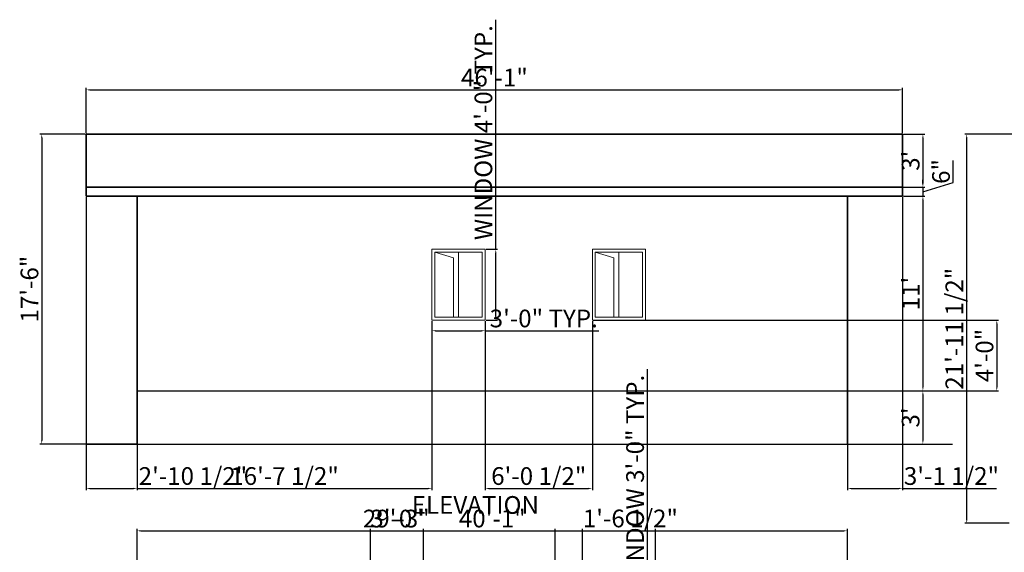
# Model space of a CAD drawing. Units: inches. Extents: x 2319 to 3765, y 2872 to 3950.
# Tile 8 of 9: x 2395 to 3061, y 3589 to 3950. Entities that reach past the tile are written whole.
import ezdxf

# ---------------------------------------------------------------- set-up
doc = ezdxf.new("R2010")
doc.units = ezdxf.units.IN
for name, color, linetype, lineweight in [('A-ANNO-DIMS', 2, 'Continuous', 18), ('A-ANNO-TEXT', 7, 'Continuous', 25), ('A-ELEV', 7, 'Continuous', 25), ('A-GLAZ', 4, 'Continuous', 18), ('A-ROOF', 7, 'Continuous', 35)]:
    doc.layers.add(name, color=color, linetype=linetype, lineweight=lineweight)
doc.styles.get("Standard").update_dxf_attribs({"font": 'arial.ttf'})
doc.dimstyles.new('ISO-25', dxfattribs={"dimtxt": 12, "dimasz": 2.5, "dimexe": 1.25, "dimexo": 0.625, "dimtad": 1, "dimdec": 0, "dimlunit": 3, "dimtxsty": 'Standard', "dimcen": 2.5, "dimadec": 0, "dimazin": 0, "dimtfac": 1, "dimtdec": 0, "dimtmove": 0, "dimatfit": 3, "dimfxl": 1, "dimarcsym": 0})

# ---------------------------------------------------------------- blocks, each defined once
blk = doc.blocks.new('*D27')
at = {"layer": 'A-ANNO-DIMS', "color": 0, "lineweight": -2, "transparency": 16777216}
for p, q in [((2993.13, 3872.56), (3007.48, 3872.56)), ((3006.23, 3870.06), (3006.23, 3839.06)), ((2993.13, 3836.56), (3007.48, 3836.56))]:
    blk.add_line(p, q, dxfattribs=at)
at = {"layer": 'A-ANNO-DIMS', "color": 0, "transparency": 16777216}
for points in [[(3005.82, 3870.06), (3006.65, 3870.06), (3006.23, 3872.56)], [(3005.82, 3839.06), (3006.65, 3839.06), (3006.23, 3836.56)]]:
    blk.add_solid(points, dxfattribs=at)
at = {"layer": 'Defpoints', "color": 0, "transparency": 16777216}
for p in [(2992.5, 3872.56), (2992.5, 3836.56), (3006.23, 3836.56)]:
    blk.add_point(p, dxfattribs=at)
at = {"layer": 'A-ANNO-DIMS', "color": 0, "transparency": 16777216, "insert": (2999.48, 3854.56), "char_height": 12, "attachment_point": 5, "rotation": 90}
blk.add_mtext("3'", dxfattribs=at)
blk = doc.blocks.new('*D28')
at = {"layer": 'A-ANNO-DIMS', "color": 0, "lineweight": -2, "transparency": 16777216}
for p, q in [((3026.8, 3839.73), (3026.8, 3854.84)), ((3006.23, 3839.06), (3006.23, 3841.56)), ((2993.13, 3836.56), (3007.48, 3836.56)), ((3006.23, 3833.56), (3026.8, 3839.73)), ((3006.23, 3836.56), (3006.23, 3830.56)), ((3006.23, 3836.56), (3006.23, 3830.56)), ((2993.13, 3830.56), (3007.48, 3830.56)), ((3006.23, 3828.06), (3006.23, 3825.56))]:
    blk.add_line(p, q, dxfattribs=at)
at = {"layer": 'A-ANNO-DIMS', "color": 0, "transparency": 16777216}
for points in [[(3005.82, 3839.06), (3006.65, 3839.06), (3006.23, 3836.56)], [(3005.82, 3828.06), (3006.65, 3828.06), (3006.23, 3830.56)]]:
    blk.add_solid(points, dxfattribs=at)
at = {"layer": 'Defpoints', "color": 0, "transparency": 16777216}
for p in [(2992.5, 3836.56), (2992.5, 3830.56), (3006.23, 3830.56)]:
    blk.add_point(p, dxfattribs=at)
at = {"layer": 'A-ANNO-DIMS', "color": 0, "transparency": 16777216, "insert": (3020.05, 3847.29), "char_height": 12, "attachment_point": 5, "rotation": 90}
blk.add_mtext('6"', dxfattribs=at)
blk = doc.blocks.new('*D29')
at = {"layer": 'A-ANNO-DIMS', "color": 0, "lineweight": -2, "transparency": 16777216}
for p, q in [((2993.13, 3830.56), (3007.48, 3830.56)), ((3006.23, 3828.06), (3006.23, 3701.06)), ((2955.75, 3698.56), (3007.48, 3698.56))]:
    blk.add_line(p, q, dxfattribs=at)
at = {"layer": 'A-ANNO-DIMS', "color": 0, "transparency": 16777216}
for points in [[(3005.82, 3828.06), (3006.65, 3828.06), (3006.23, 3830.56)], [(3005.82, 3701.06), (3006.65, 3701.06), (3006.23, 3698.56)]]:
    blk.add_solid(points, dxfattribs=at)
at = {"layer": 'Defpoints', "color": 0, "transparency": 16777216}
for p in [(2992.5, 3830.56), (2955.13, 3698.56), (3006.23, 3698.56)]:
    blk.add_point(p, dxfattribs=at)
at = {"layer": 'A-ANNO-DIMS', "color": 0, "transparency": 16777216, "insert": (2999.58, 3764.56), "char_height": 12, "attachment_point": 5, "rotation": 90}
blk.add_mtext("11'", dxfattribs=at)
blk = doc.blocks.new('*D30')
at = {"layer": 'A-ANNO-DIMS', "color": 0, "lineweight": -2, "transparency": 16777216}
for p, q in [((2955.75, 3698.56), (3007.48, 3698.56)), ((3006.23, 3696.06), (3006.23, 3665.06)), ((2955.75, 3662.56), (3007.48, 3662.56))]:
    blk.add_line(p, q, dxfattribs=at)
at = {"layer": 'A-ANNO-DIMS', "color": 0, "transparency": 16777216}
for points in [[(3005.82, 3696.06), (3006.65, 3696.06), (3006.23, 3698.56)], [(3005.82, 3665.06), (3006.65, 3665.06), (3006.23, 3662.56)]]:
    blk.add_solid(points, dxfattribs=at)
at = {"layer": 'Defpoints', "color": 0, "transparency": 16777216}
for p in [(2955.13, 3698.56), (2955.13, 3662.56), (3006.23, 3662.56)]:
    blk.add_point(p, dxfattribs=at)
at = {"layer": 'A-ANNO-DIMS', "color": 0, "transparency": 16777216, "insert": (2999.48, 3680.56), "char_height": 12, "attachment_point": 5, "rotation": 90}
blk.add_mtext("3'", dxfattribs=at)
blk = doc.blocks.new('WIN-36X48-ELEV')
for p, q in [((2, 46), (14.59, 42.21)), ((14.59, 42.21), (14.59, 2.09)), ((18, 2), (18, 46))]:
    blk.add_line(p, q)
for points in [[(0, 0), (36, 0), (36, 48), (0, 48)], [(2, 2), (34, 2), (34, 46), (2, 46)]]:
    blk.add_lwpolyline(points, close=True)
blk = doc.blocks.new('*D61')
at = {"layer": 'A-ANNO-DIMS', "color": 0, "lineweight": -2, "transparency": 16777216}
for p, q in [((2819.73, 3557.62), (2819.73, 3713.22)), ((2824.5, 3557.62), (2818.48, 3557.62)), ((2819.73, 3524.12), (2819.73, 3555.12)), ((2824.5, 3521.62), (2818.48, 3521.62))]:
    blk.add_line(p, q, dxfattribs=at)
at = {"layer": 'A-ANNO-DIMS', "color": 0, "transparency": 16777216}
for points in [[(2819.31, 3555.12), (2820.14, 3555.12), (2819.73, 3557.62)], [(2819.31, 3524.12), (2820.14, 3524.12), (2819.73, 3521.62)]]:
    blk.add_solid(points, dxfattribs=at)
at = {"layer": 'Defpoints', "color": 0, "transparency": 16777216}
for p in [(2819.73, 3557.62), (2825.13, 3557.62), (2825.13, 3521.62)]:
    blk.add_point(p, dxfattribs=at)
at = {"layer": 'A-ANNO-DIMS', "color": 0, "transparency": 16777216, "insert": (2812.89, 3636.67), "char_height": 12, "attachment_point": 5, "rotation": 90}
blk.add_mtext('WINDOW 3\'-0" TYP.', dxfattribs=at)
blk = doc.blocks.new('*D67')
at = {"layer": 'A-ANNO-DIMS', "color": 0, "lineweight": -2, "transparency": 16777216}
for p, q in [((2717.01, 3794.56), (2717.01, 3950.16)), ((2710.44, 3794.56), (2718.26, 3794.56)), ((2717.01, 3749.06), (2717.01, 3792.06)), ((2710.44, 3746.56), (2718.26, 3746.56))]:
    blk.add_line(p, q, dxfattribs=at)
at = {"layer": 'A-ANNO-DIMS', "color": 0, "transparency": 16777216}
for points in [[(2716.6, 3792.06), (2717.43, 3792.06), (2717.01, 3794.56)], [(2716.6, 3749.06), (2717.43, 3749.06), (2717.01, 3746.56)]]:
    blk.add_solid(points, dxfattribs=at)
at = {"layer": 'Defpoints', "color": 0, "transparency": 16777216}
for p in [(2709.81, 3794.56), (2717.01, 3794.56), (2709.81, 3746.56)]:
    blk.add_point(p, dxfattribs=at)
at = {"layer": 'A-ANNO-DIMS', "color": 0, "transparency": 16777216, "insert": (2710.18, 3873.61), "char_height": 12, "attachment_point": 5, "rotation": 90}
blk.add_mtext('WINDOW 4\'-0" TYP.', dxfattribs=at)
blk = doc.blocks.new('*D68')
at = {"layer": 'A-ANNO-DIMS', "color": 0, "lineweight": -2, "transparency": 16777216}
for p, q in [((2673.81, 3745.94), (2673.81, 3738.11)), ((2709.81, 3745.94), (2709.81, 3738.11)), ((2676.31, 3739.36), (2707.31, 3739.36)), ((2709.81, 3739.36), (2786.7, 3739.36))]:
    blk.add_line(p, q, dxfattribs=at)
at = {"layer": 'A-ANNO-DIMS', "color": 0, "transparency": 16777216}
for points in [[(2676.31, 3739.78), (2676.31, 3738.94), (2673.81, 3739.36)], [(2707.31, 3739.78), (2707.31, 3738.94), (2709.81, 3739.36)]]:
    blk.add_solid(points, dxfattribs=at)
at = {"layer": 'Defpoints', "color": 0, "transparency": 16777216}
for p in [(2673.81, 3746.56), (2709.81, 3746.56), (2709.81, 3739.36)]:
    blk.add_point(p, dxfattribs=at)
at = {"layer": 'A-ANNO-DIMS', "color": 0, "transparency": 16777216, "insert": (2749.51, 3746.12), "char_height": 12, "attachment_point": 5}
blk.add_mtext('3\'-0" TYP.', dxfattribs=at)
blk = doc.blocks.new('*D71')
at = {"layer": 'A-ANNO-DIMS', "color": 0, "lineweight": -2, "transparency": 16777216}
for p, q in [((2474.13, 3507.24), (2474.13, 3605.01)), ((2476.63, 3603.76), (2952.63, 3603.76)), ((2955.13, 3569.24), (2955.13, 3605.01))]:
    blk.add_line(p, q, dxfattribs=at)
at = {"layer": 'A-ANNO-DIMS', "color": 0, "transparency": 16777216}
for points in [[(2476.63, 3604.18), (2476.63, 3603.34), (2474.13, 3603.76)], [(2952.63, 3604.18), (2952.63, 3603.34), (2955.13, 3603.76)]]:
    blk.add_solid(points, dxfattribs=at)
at = {"layer": 'Defpoints', "color": 0, "transparency": 16777216}
for p in [(2955.13, 3603.76), (2955.13, 3568.61), (2474.13, 3506.61)]:
    blk.add_point(p, dxfattribs=at)
at = {"layer": 'A-ANNO-DIMS', "color": 0, "transparency": 16777216, "insert": (2714.63, 3610.51), "char_height": 12, "attachment_point": 5}
blk.add_mtext('40\'-1"', dxfattribs=at)
blk = doc.blocks.new('*D73')
at = {"layer": 'A-ANNO-DIMS', "color": 0, "lineweight": -2, "transparency": 16777216}
for p, q in [((2474.13, 3507.24), (2474.13, 3605.01)), ((2476.63, 3603.76), (2822.63, 3603.76)), ((2825.13, 3507.24), (2825.13, 3605.01))]:
    blk.add_line(p, q, dxfattribs=at)
at = {"layer": 'A-ANNO-DIMS', "color": 0, "transparency": 16777216}
for points in [[(2476.63, 3604.18), (2476.63, 3603.34), (2474.13, 3603.76)], [(2822.63, 3604.18), (2822.63, 3603.34), (2825.13, 3603.76)]]:
    blk.add_solid(points, dxfattribs=at)
at = {"layer": 'Defpoints', "color": 0, "transparency": 16777216}
for p in [(2825.13, 3603.76), (2474.13, 3506.61), (2825.13, 3506.61)]:
    blk.add_point(p, dxfattribs=at)
at = {"layer": 'A-ANNO-DIMS', "color": 0, "transparency": 16777216, "insert": (2649.63, 3610.52), "char_height": 12, "attachment_point": 5}
blk.add_mtext('29\'-3"', dxfattribs=at)
blk = doc.blocks.new('*D75')
at = {"layer": 'A-ANNO-DIMS', "color": 0, "lineweight": -2, "transparency": 16777216}
for p, q in [((2632.13, 2970.24), (2632.13, 3605.01)), ((2634.63, 3603.76), (2665.63, 3603.76)), ((2668.13, 2970.24), (2668.13, 3605.01))]:
    blk.add_line(p, q, dxfattribs=at)
at = {"layer": 'A-ANNO-DIMS', "color": 0, "transparency": 16777216}
for points in [[(2634.63, 3604.18), (2634.63, 3603.34), (2632.13, 3603.76)], [(2665.63, 3604.18), (2665.63, 3603.34), (2668.13, 3603.76)]]:
    blk.add_solid(points, dxfattribs=at)
at = {"layer": 'Defpoints', "color": 0, "transparency": 16777216}
for p in [(2668.13, 3603.76), (2632.13, 2969.61), (2668.13, 2969.61)]:
    blk.add_point(p, dxfattribs=at)
at = {"layer": 'A-ANNO-DIMS', "color": 0, "transparency": 16777216, "insert": (2650.13, 3610.52), "char_height": 12, "attachment_point": 5}
blk.add_mtext('3\'-0"', dxfattribs=at)
blk = doc.blocks.new('*D76')
at = {"layer": 'A-ANNO-DIMS', "color": 0, "lineweight": -2, "transparency": 16777216}
for p, q in [((2757.13, 2970.24), (2757.13, 3605.01)), ((2759.63, 3603.76), (2773.17, 3603.76)), ((2775.67, 2970.24), (2775.67, 3605.01)), ((2775.67, 3603.76), (2838.15, 3603.76))]:
    blk.add_line(p, q, dxfattribs=at)
at = {"layer": 'A-ANNO-DIMS', "color": 0, "transparency": 16777216}
for points in [[(2759.63, 3604.18), (2759.63, 3603.34), (2757.13, 3603.76)], [(2773.17, 3604.18), (2773.17, 3603.34), (2775.67, 3603.76)]]:
    blk.add_solid(points, dxfattribs=at)
at = {"layer": 'Defpoints', "color": 0, "transparency": 16777216}
for p in [(2775.67, 3603.76), (2757.13, 2969.61), (2775.67, 2969.61)]:
    blk.add_point(p, dxfattribs=at)
at = {"layer": 'A-ANNO-DIMS', "color": 0, "transparency": 16777216, "insert": (2808.16, 3610.59), "char_height": 12, "attachment_point": 5}
blk.add_mtext('1\'-6 1/2"', dxfattribs=at)
blk = doc.blocks.new('*D89')
at = {"layer": 'A-ANNO-DIMS', "color": 0, "lineweight": -2, "transparency": 16777216}
for p, q in [((2439.63, 3873.19), (2439.63, 3903.86)), ((2442.13, 3902.61), (2990, 3902.61)), ((2992.5, 3873.19), (2992.5, 3903.86))]:
    blk.add_line(p, q, dxfattribs=at)
at = {"layer": 'A-ANNO-DIMS', "color": 0, "transparency": 16777216}
for points in [[(2442.13, 3903.03), (2442.13, 3902.19), (2439.63, 3902.61)], [(2990, 3903.03), (2990, 3902.19), (2992.5, 3902.61)]]:
    blk.add_solid(points, dxfattribs=at)
at = {"layer": 'Defpoints', "color": 0, "transparency": 16777216}
for p in [(2992.5, 3902.61), (2439.63, 3872.56), (2992.5, 3872.56)]:
    blk.add_point(p, dxfattribs=at)
at = {"layer": 'A-ANNO-DIMS', "color": 0, "transparency": 16777216, "insert": (2716.07, 3909.36), "char_height": 12, "attachment_point": 5}
blk.add_mtext('46\'-1"', dxfattribs=at)
blk = doc.blocks.new('*D90')
at = {"layer": 'A-ANNO-DIMS', "color": 0, "lineweight": -2, "transparency": 16777216}
for p, q in [((2439, 3872.56), (2408.33, 3872.56)), ((2409.58, 3870.06), (2409.58, 3665.06)), ((2473.5, 3662.56), (2408.33, 3662.56))]:
    blk.add_line(p, q, dxfattribs=at)
at = {"layer": 'A-ANNO-DIMS', "color": 0, "transparency": 16777216}
for points in [[(2409.16, 3870.06), (2409.99, 3870.06), (2409.58, 3872.56)], [(2409.16, 3665.06), (2409.99, 3665.06), (2409.58, 3662.56)]]:
    blk.add_solid(points, dxfattribs=at)
at = {"layer": 'Defpoints', "color": 0, "transparency": 16777216}
for p in [(2439.63, 3872.56), (2409.58, 3662.56), (2474.13, 3662.56)]:
    blk.add_point(p, dxfattribs=at)
at = {"layer": 'A-ANNO-DIMS', "color": 0, "transparency": 16777216, "insert": (2402.83, 3767.56), "char_height": 12, "attachment_point": 5, "rotation": 90}
blk.add_mtext('17\'-6"', dxfattribs=at)
blk = doc.blocks.new('*D91')
at = {"layer": 'A-ANNO-DIMS', "color": 0, "lineweight": -2, "transparency": 16777216}
for p, q in [((2439.63, 3829.94), (2439.63, 3631.26)), ((2474.13, 3829.94), (2474.13, 3631.26)), ((2442.13, 3632.51), (2471.63, 3632.51)), ((2474.13, 3632.51), (2547.27, 3632.51))]:
    blk.add_line(p, q, dxfattribs=at)
at = {"layer": 'A-ANNO-DIMS', "color": 0, "transparency": 16777216}
for points in [[(2442.13, 3632.93), (2442.13, 3632.09), (2439.63, 3632.51)], [(2471.63, 3632.93), (2471.63, 3632.09), (2474.13, 3632.51)]]:
    blk.add_solid(points, dxfattribs=at)
at = {"layer": 'Defpoints', "color": 0, "transparency": 16777216}
for p in [(2439.63, 3830.56), (2474.13, 3830.56), (2474.13, 3632.51)]:
    blk.add_point(p, dxfattribs=at)
at = {"layer": 'A-ANNO-DIMS', "color": 0, "transparency": 16777216, "insert": (2511.95, 3639.34), "char_height": 12, "attachment_point": 5}
blk.add_mtext('2\'-10 1/2"', dxfattribs=at)
blk = doc.blocks.new('*D92')
at = {"layer": 'A-ANNO-DIMS', "color": 0, "lineweight": -2, "transparency": 16777216}
for p, q in [((2955.13, 3829.94), (2955.13, 3631.26)), ((2992.5, 3829.94), (2992.5, 3631.26)), ((2957.63, 3632.51), (2990, 3632.51)), ((2992.5, 3632.51), (3056.11, 3632.51))]:
    blk.add_line(p, q, dxfattribs=at)
at = {"layer": 'A-ANNO-DIMS', "color": 0, "transparency": 16777216}
for points in [[(2957.63, 3632.93), (2957.63, 3632.09), (2955.13, 3632.51)], [(2990, 3632.93), (2990, 3632.09), (2992.5, 3632.51)]]:
    blk.add_solid(points, dxfattribs=at)
at = {"layer": 'Defpoints', "color": 0, "transparency": 16777216}
for p in [(2955.13, 3830.56), (2992.5, 3830.56), (2992.5, 3632.51)]:
    blk.add_point(p, dxfattribs=at)
at = {"layer": 'A-ANNO-DIMS', "color": 0, "transparency": 16777216, "insert": (3025.56, 3639.34), "char_height": 12, "attachment_point": 5}
blk.add_mtext('3\'-1 1/2"', dxfattribs=at)
blk = doc.blocks.new('*D93')
at = {"layer": 'A-ANNO-DIMS', "color": 0, "lineweight": -2, "transparency": 16777216}
for p, q in [((2673.81, 3745.94), (2673.81, 3631.26)), ((2474.13, 3697.94), (2474.13, 3631.26)), ((2476.63, 3632.51), (2671.31, 3632.51))]:
    blk.add_line(p, q, dxfattribs=at)
at = {"layer": 'A-ANNO-DIMS', "color": 0, "transparency": 16777216}
for points in [[(2476.63, 3632.93), (2476.63, 3632.09), (2474.13, 3632.51)], [(2671.31, 3632.93), (2671.31, 3632.09), (2673.81, 3632.51)]]:
    blk.add_solid(points, dxfattribs=at)
at = {"layer": 'Defpoints', "color": 0, "transparency": 16777216}
for p in [(2673.81, 3746.56), (2474.13, 3698.56), (2673.81, 3632.51)]:
    blk.add_point(p, dxfattribs=at)
at = {"layer": 'A-ANNO-DIMS', "color": 0, "transparency": 16777216, "insert": (2573.97, 3639.34), "char_height": 12, "attachment_point": 5}
blk.add_mtext('16\'-7 1/2"', dxfattribs=at)
blk = doc.blocks.new('*D94')
at = {"layer": 'A-ANNO-DIMS', "color": 0, "lineweight": -2, "transparency": 16777216}
for p, q in [((2709.81, 3745.94), (2709.81, 3631.26)), ((2782.41, 3745.94), (2782.41, 3631.26)), ((2712.31, 3632.51), (2779.91, 3632.51))]:
    blk.add_line(p, q, dxfattribs=at)
at = {"layer": 'A-ANNO-DIMS', "color": 0, "transparency": 16777216}
for points in [[(2712.31, 3632.93), (2712.31, 3632.09), (2709.81, 3632.51)], [(2779.91, 3632.93), (2779.91, 3632.09), (2782.41, 3632.51)]]:
    blk.add_solid(points, dxfattribs=at)
at = {"layer": 'Defpoints', "color": 0, "transparency": 16777216}
for p in [(2709.81, 3746.56), (2782.41, 3746.56), (2782.41, 3632.51)]:
    blk.add_point(p, dxfattribs=at)
at = {"layer": 'A-ANNO-DIMS', "color": 0, "transparency": 16777216, "insert": (2746.11, 3639.34), "char_height": 12, "attachment_point": 5}
blk.add_mtext('6\'-0 1/2"', dxfattribs=at)
blk = doc.blocks.new('*D95')
at = {"layer": 'A-ANNO-DIMS', "color": 0, "lineweight": -2, "transparency": 16777216}
for p, q in [((2783.03, 3746.56), (3057.51, 3746.56)), ((3056.26, 3744.06), (3056.26, 3701.06)), ((2955.75, 3698.56), (3057.51, 3698.56))]:
    blk.add_line(p, q, dxfattribs=at)
at = {"layer": 'A-ANNO-DIMS', "color": 0, "transparency": 16777216}
for points in [[(3055.84, 3744.06), (3056.67, 3744.06), (3056.26, 3746.56)], [(3055.84, 3701.06), (3056.67, 3701.06), (3056.26, 3698.56)]]:
    blk.add_solid(points, dxfattribs=at)
at = {"layer": 'Defpoints', "color": 0, "transparency": 16777216}
for p in [(2782.41, 3746.56), (2955.13, 3698.56), (3056.26, 3698.56)]:
    blk.add_point(p, dxfattribs=at)
at = {"layer": 'A-ANNO-DIMS', "color": 0, "transparency": 16777216, "insert": (3049.5, 3722.56), "char_height": 12, "attachment_point": 5, "rotation": 90}
blk.add_mtext('4\'-0"', dxfattribs=at)
blk = doc.blocks.new('*D97')
at = {"layer": 'A-ANNO-DIMS', "color": 0, "lineweight": -2, "transparency": 16777216}
for p, q in [((3077.94, 3872.56), (3034.65, 3872.56)), ((3035.9, 3611.36), (3035.9, 3870.06)), ((3064.57, 3608.86), (3034.65, 3608.86))]:
    blk.add_line(p, q, dxfattribs=at)
at = {"layer": 'A-ANNO-DIMS', "color": 0, "transparency": 16777216}
for points in [[(3035.48, 3870.06), (3036.31, 3870.06), (3035.9, 3872.56)], [(3035.48, 3611.36), (3036.31, 3611.36), (3035.9, 3608.86)]]:
    blk.add_solid(points, dxfattribs=at)
at = {"layer": 'Defpoints', "color": 0, "transparency": 16777216}
for p in [(3035.9, 3872.56), (3078.57, 3872.56), (3065.2, 3608.86)]:
    blk.add_point(p, dxfattribs=at)
at = {"layer": 'A-ANNO-DIMS', "color": 0, "transparency": 16777216, "insert": (3029.07, 3740.71), "char_height": 12, "attachment_point": 5, "rotation": 90}
blk.add_mtext('21\'-11 1/2"', dxfattribs=at)

msp = doc.modelspace()

# ---------------------------------------------------------------- linework, layer by layer
at = {"layer": 'A-ELEV'}
for p, q in [((2474.13, 3662.56), (2474.13, 3830.56)), ((2955.13, 3662.56), (2955.13, 3830.56)), ((2474.13, 3698.56), (2955.13, 3698.56)), ((2439.63, 3662.56), (3026.21, 3662.56))]:
    msp.add_line(p, q, dxfattribs=at)
at = {"layer": 'A-ROOF'}
for p, q in [((2439.63, 3872.56), (2992.5, 3872.56)), ((2439.63, 3830.56), (2439.63, 3872.56)), ((2992.5, 3830.56), (2992.5, 3872.56)), ((2439.63, 3836.56), (2992.5, 3836.56)), ((2439.63, 3830.56), (2992.5, 3830.56))]:
    msp.add_line(p, q, dxfattribs=at)

# ---------------------------------------------------------------- block references
at = {"layer": 'A-GLAZ'}
for p in [(2673.81, 3746.56), (2782.41, 3746.56)]:
    msp.add_blockref('WIN-36X48-ELEV', p, dxfattribs=at)

# ---------------------------------------------------------------- texts
at = {"layer": 'A-ANNO-TEXT'}
msp.add_text('ELEVATION', height=12, dxfattribs=at).set_placement((2660.13, 3615.29))

# ---------------------------------------------------------------- dimensions: what is measured, and where the dimension line sits
at = {"layer": 'A-ANNO-DIMS'}
for base, p1, p2, picture, middle in [((2717.01, 3794.56), (2709.81, 3746.56), (2709.81, 3794.56), '*D67', (2710.18, 3873.61)), ((2819.73, 3557.62), (2825.13, 3521.62), (2825.13, 3557.62), '*D61', (2812.89, 3636.67))]:
    dim = msp.add_linear_dim(base=base, p1=p1, p2=p2, angle=90, text='WINDOW <> TYP.', dimstyle='ISO-25', override={"dimdec": 1, "dimlfac": 1, "dimrnd": 0, "dimzin": 1, "dimdsep": 46, "dimlunit": 4, "dimfrac": 2}, dxfattribs=at)
    dim.commit()
    dim.dimension.update_dxf_attribs({"geometry": picture, "text_midpoint": middle})
for base, p1, p2, picture, middle in [((2992.5, 3902.61), (2439.63, 3872.56), (2992.5, 3872.56), '*D89', (2716.07, 3909.36)), ((2474.13, 3632.51), (2439.63, 3830.56), (2474.13, 3830.56), '*D91', (2511.95, 3639.34)), ((2992.5, 3632.51), (2955.13, 3830.56), (2992.5, 3830.56), '*D92', (3025.56, 3639.34)), ((2673.81, 3632.51), (2474.13, 3698.56), (2673.81, 3746.56), '*D93', (2573.97, 3639.34)), ((2782.41, 3632.51), (2709.81, 3746.56), (2782.41, 3746.56), '*D94', (2746.11, 3639.34)), ((2775.67, 3603.76), (2757.13, 2969.61), (2775.67, 2969.61), '*D76', (2808.16, 3610.59)), ((2955.13, 3603.76), (2474.13, 3506.61), (2955.13, 3568.61), '*D71', (2714.63, 3610.51)), ((2825.13, 3603.76), (2474.13, 3506.61), (2825.13, 3506.61), '*D73', (2649.63, 3610.52)), ((2668.13, 3603.76), (2632.13, 2969.61), (2668.13, 2969.61), '*D75', (2650.13, 3610.52))]:
    dim = msp.add_linear_dim(base=base, p1=p1, p2=p2, dimstyle='ISO-25', override={"dimdec": 1, "dimlfac": 1, "dimrnd": 0, "dimzin": 1, "dimdsep": 46, "dimlunit": 4, "dimfrac": 2}, dxfattribs=at)
    dim.commit()
    dim.dimension.update_dxf_attribs({"geometry": picture, "text_midpoint": middle})
for base, p1, p2, override, picture, middle in [((2409.58, 3662.56), (2439.63, 3872.56), (2474.13, 3662.56), {"dimdec": 1, "dimlfac": 1, "dimrnd": 0, "dimzin": 1, "dimdsep": 46, "dimlunit": 4, "dimfrac": 2}, '*D90', (2402.83, 3767.56)), ((3006.23, 3836.56), (2992.5, 3872.56), (2992.5, 3836.56), {"dimclrd": 0, "dimclre": 0, "dimclrt": 0}, '*D27', (2999.48, 3854.56)), ((3035.9, 3872.56), (3065.2, 3608.86), (3078.57, 3872.56), {"dimdec": 1, "dimlfac": 1, "dimrnd": 0, "dimzin": 1, "dimdsep": 46, "dimlunit": 4, "dimfrac": 2}, '*D97', (3029.07, 3740.71)), ((3006.23, 3830.56), (2992.5, 3836.56), (2992.5, 3830.56), {"dimclrd": 0, "dimclre": 0, "dimclrt": 0, "dimtmove": 1}, '*D28', (3020.05, 3840.36)), ((3006.23, 3698.56), (2992.5, 3830.56), (2955.13, 3698.56), {"dimclrd": 0, "dimclre": 0, "dimclrt": 0, "dimtmove": 1}, '*D29', (2999.58, 3764.56)), ((3056.26, 3698.56), (2782.41, 3746.56), (2955.13, 3698.56), {"dimdec": 1, "dimlfac": 1, "dimrnd": 0, "dimzin": 1, "dimdsep": 46, "dimlunit": 4, "dimfrac": 2}, '*D95', (3049.5, 3722.56)), ((3006.23, 3662.56), (2955.13, 3698.56), (2955.13, 3662.56), {"dimclrd": 0, "dimclre": 0, "dimclrt": 0, "dimtmove": 1}, '*D30', (2999.48, 3680.56))]:
    dim = msp.add_linear_dim(base=base, p1=p1, p2=p2, angle=90, dimstyle='ISO-25', override=override, dxfattribs=at)
    dim.commit()
    dim.dimension.update_dxf_attribs({"geometry": picture, "text_midpoint": middle})
dim = msp.add_linear_dim(base=(2709.81, 3739.36), p1=(2673.81, 3746.56), p2=(2709.81, 3746.56), text='<> TYP.', dimstyle='ISO-25', override={"dimdec": 1, "dimlfac": 1, "dimrnd": 0, "dimzin": 1, "dimdsep": 46, "dimlunit": 4, "dimfrac": 2}, dxfattribs=at)
dim.commit()
dim.dimension.update_dxf_attribs({"geometry": '*D68', "text_midpoint": (2749.51, 3746.12)})

doc.saveas('drawing.dxf')
